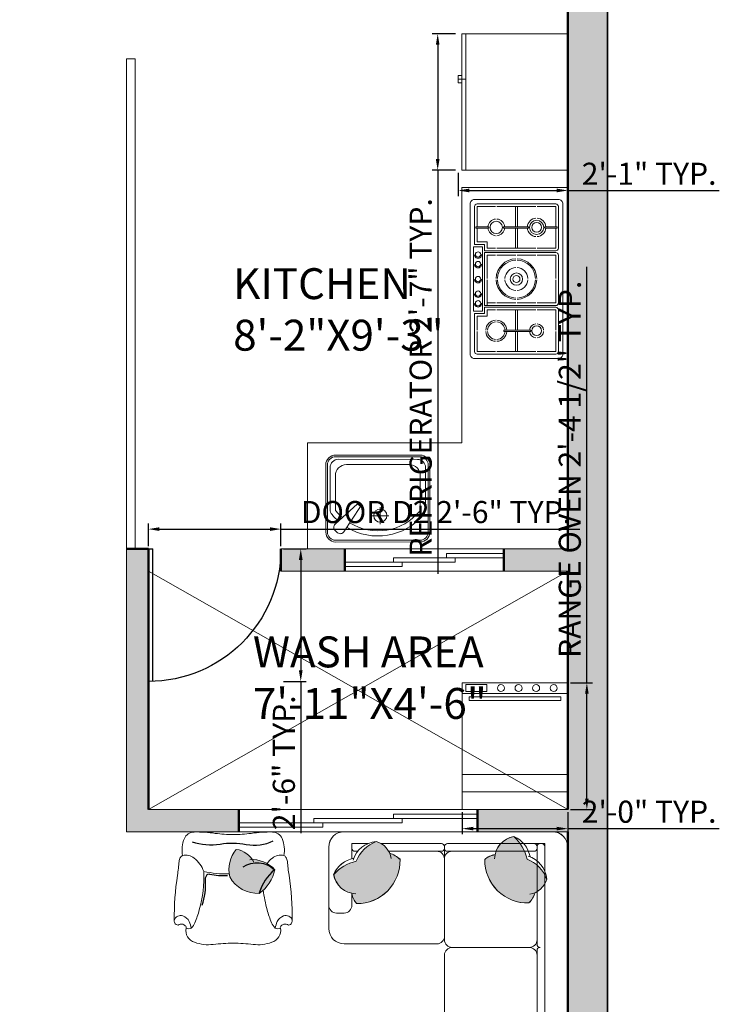
# Model space of a CAD drawing. Units: inches. Extents: x 1734 to 4011, y 1071 to 1891.
# Tile 4 of 27: x 1985 to 2144, y 1427 to 1650. Entities that reach past the tile are written whole.
import ezdxf

# ---------------------------------------------------------------- set-up
doc = ezdxf.new("R2010")
doc.units = ezdxf.units.IN
for name, color, linetype, lineweight in [('A-ANNO-DIMS', 2, 'Continuous', 18), ('A-AREA-IDEN', 3, 'Continuous', 18), ('A-DOOR', 3, 'Continuous', 25), ('A-EQPM', 8, 'Continuous', 18), ('A-FLOR-FIXT', 9, 'Continuous', 18), ('A-FURN', 8, 'Continuous', 18), ('A-FURN-PATT', 252, 'Continuous', 13), ('A-GLAZ', 4, 'Continuous', 18), ('A-WALL', 7, 'Continuous', 50), ('A-WALL-PATT', 8, 'Continuous', 13), ('C-PROP', 1, 'Continuous', 35)]:
    doc.layers.add(name, color=color, linetype=linetype, lineweight=lineweight)
doc.layers.add('IFF-FURN-DETAIL', color=250, linetype='Continuous')
doc.styles.get("Standard").update_dxf_attribs({"font": 'arial.ttf'})
doc.dimstyles.new('ISO-25', dxfattribs={"dimtxt": 5, "dimasz": 2.5, "dimexe": 1.25, "dimexo": 0.625, "dimtad": 1, "dimdec": 1, "dimlunit": 3, "dimtxsty": 'Standard', "dimcen": 2.5, "dimclrt": 1, "dimadec": 0, "dimazin": 0, "dimtfac": 1, "dimtdec": 1, "dimtmove": 0, "dimatfit": 3, "dimfxl": 1, "dimarcsym": 0})

# ---------------------------------------------------------------- blocks, each defined once
blk = doc.blocks.new('STOVE')
for p, q in [((11.85, 19.7), (11.55, 19.7)), ((11.55, 16.92), (11.55, 19.7)), ((11.85, 16.92), (11.85, 19.7)), ((11.85, 16.92), (11.55, 16.92)), ((-11.85, 13.73), (-11.85, 7.62)), ((-11.85, 13.73), (-11.55, 13.73)), ((-11.55, 13.73), (-11.55, 7.62)), ((11.85, 13.23), (11.55, 13.23)), ((11.55, 13.23), (11.55, 7.57)), ((11.85, 13.23), (11.85, 7.57)), ((-11.85, 10.75), (-16.4, 10.75)), ((-11.85, 10.25), (-16.4, 10.25)), ((-7, 10.75), (-11.55, 10.75)), ((-7, 10.25), (-11.55, 10.25)), ((7, 10.75), (11.55, 10.75)), ((7, 10.25), (11.55, 10.25)), ((11.85, 10.75), (16.4, 10.75)), ((11.85, 10.25), (16.4, 10.25)), ((-11.85, 7.62), (-11.55, 7.62)), ((11.85, 7.57), (11.55, 7.57)), ((-7, 3.9), (-8.4, 3.9)), ((-7.8, 3.3), (-7.8, 1)), ((-6.4, 3.3), (-7.8, 3.3)), ((7.3, 2.8), (-7.3, 2.8)), ((-7.3, 2.8), (-7.3, 0.8)), ((-5.4, 3.9), (-6, 3.9)), ((-5.4, 3.9), (-0.15, 3.9)), ((0.15, 3.9), (5.4, 3.9)), ((6.4, 3.3), (7.8, 3.3)), ((7, 3.9), (8.4, 3.9)), ((7.3, 2.8), (7.3, 0.8)), ((7.8, 3.3), (7.8, 1)), ((8.4, 3.9), (8.4, 1.6)), ((11.85, 4.28), (11.55, 4.28)), ((11.55, 4.28), (11.55, 1.3)), ((11.85, 4.28), (11.85, 1.3)), ((7.3, 0.8), (-7.3, 0.8)), ((11.85, 1.3), (11.55, 1.3))]:
    blk.add_line(p, q)
for points in [[(-17, 21), (17, 21, -0.414214), (18, 20), (18, 1, -0.414214), (17, 0), (-17, 0, -0.414214), (-18, 1), (-18, 20, -0.414214)], [(6, 3.3), (-6, 3.3), (-6, 19.4, -0.414214), (-5.4, 20), (5.4, 20, -0.414214), (6, 19.4)]]:
    blk.add_lwpolyline(points, format="xyb", close=True)
for points in [[(-7.8, 1), (-16.4, 1, -0.414214), (-17, 1.6), (-17, 19.4, -0.414214), (-16.4, 20), (-7, 20, -0.414214), (-6.4, 19.4), (-6.4, 3.3)], [(6.4, 19.4, -0.414214), (7, 20), (16.4, 20, -0.414214), (17, 19.4), (17, 1.6, -0.414214), (16.4, 1), (7.8, 1)]]:
    blk.add_lwpolyline(points, format="xyb")
for points in [[(-16.4, 15.22), (-16.4, 19.4), (-11.85, 19.4)], [(-11.55, 19.4), (-7, 19.4), (-7, 15.22)], [(-5.4, 15.22), (-5.4, 19.4), (-0.15, 19.4)], [(0.15, 19.4), (5.4, 19.4), (5.4, 15.22)], [(6.4, 3.3), (6.4, 19.4)], [(7, 15.22), (7, 19.4), (11.55, 19.4)], [(11.85, 19.4), (16.4, 19.4), (16.4, 15.22)], [(-16.4, 6.08), (-16.4, 14.92)], [(-7, 14.92), (-7, 6.08)], [(-5.4, 10.65), (-5.4, 14.92)], [(5.4, 14.92), (5.4, 10.65)], [(7, 6.08), (7, 14.92)], [(16.4, 14.92), (16.4, 6.08)], [(-5.4, 6.08), (-5.4, 10.35)], [(5.4, 10.35), (5.4, 6.08)], [(-11.85, 1.6), (-16.4, 1.6), (-16.4, 5.77)], [(-7, 5.77), (-7, 3.9)], [(-5.4, 3.9), (-5.4, 5.77)], [(5.4, 5.77), (5.4, 3.9)], [(7, 3.9), (7, 5.77)], [(16.4, 5.77), (16.4, 1.6), (11.85, 1.6)], [(-8.4, 3.9), (-8.4, 1.6), (-11.55, 1.6)], [(11.55, 1.6), (8.4, 1.6)]]:
    blk.add_lwpolyline(points)
for centre, radius in [((-11.7, 15.07), 1.1), ((11.7, 15.07), 1.6), ((11.7, 15.07), 1.1), ((0, 10.5), 1.4), ((0, 10.5), 0.8), ((11.7, 5.93), 1.4), ((-5.49, 1.8), 0.6), ((-3.3, 1.8), 0.6), ((0, 1.8), 0.6), ((3.39, 1.8), 0.6), ((5.57, 1.8), 0.6)]:
    blk.add_circle(centre, radius)
for centre, radius, start, end in [((-11.7, 15.07), 1.6, 95.3794, 174.6206), ((-11.7, 15.07), 1.6, 5.3794, 84.6206), ((11.7, 15.07), 2.1, 94.096, 175.904), ((11.7, 15.07), 2.1, 4.096, 85.904), ((-11.7, 15.07), 1.6, 185.3794, 264.6206), ((-11.7, 15.07), 1.6, 275.3794, 354.6206), ((0, 10.5), 4.6, 91.8687, 178.1313), ((0, 10.5), 4.3, 91.9991, 178.0009), ((0, 10.5), 4.6, 1.8687, 88.1313), ((0, 10.5), 4.3, 1.9991, 88.0009), ((11.7, 15.07), 2.1, 184.096, 265.904), ((11.7, 15.07), 2.1, 274.096, 355.904), ((0, 10.5), 2.6, 93.3074, 176.6926), ((0, 10.5), 2.6, 3.3074, 86.6926), ((0, 10.5), 4.6, 181.8687, 268.1313), ((0, 10.5), 4.3, 181.9991, 268.0009), ((0, 10.5), 2.6, 183.3074, 266.6926), ((0, 10.5), 4.6, 271.8687, 358.1313), ((0, 10.5), 4.3, 271.9991, 358.0009), ((0, 10.5), 2.6, 273.3074, 356.6926), ((-11.7, 5.93), 2.4, 93.5833, 176.4167), ((-11.7, 5.93), 2, 94.3012, 175.6988), ((-11.7, 5.93), 2.4, 3.5833, 86.4167), ((-11.7, 5.93), 2, 4.3012, 85.6988), ((11.7, 5.93), 1.9, 94.5281, 175.4719), ((11.7, 5.93), 1.9, 4.5281, 85.4719), ((-11.7, 5.93), 2.4, 183.5833, 266.4167), ((-11.7, 5.93), 2, 184.3012, 265.6988), ((-11.7, 5.93), 2.4, 273.5833, 356.4167), ((-11.7, 5.93), 2, 274.3012, 355.6988), ((11.7, 5.93), 1.9, 184.5281, 265.4719), ((11.7, 5.93), 1.9, 274.5281, 355.4719), ((-5.49, 1.8), 0.846, 89.9979, 270), ((-3.3, 1.8), 0.846, 89.9979, 270), ((0, 1.8), 0.846, 89.9979, 270), ((3.39, 1.8), 0.846, 89.9979, 270), ((5.57, 1.8), 0.846, 89.9979, 270)]:
    blk.add_arc(centre, radius, start, end)
blk = doc.blocks.new('Refrigerator-2 door - 36 in top')
for p, q in [((0, -26.999999), (36, -26.999999)), ((11, -27.999999), (11, -28.999999)), ((12, -26.999999), (12, -28.999999)), ((13, -28.999999), (13, -27.999999)), ((11, -28.999999), (13, -28.999999))]:
    blk.add_line(p, q)
blk.add_lwpolyline([(0, -27.999999), (0, 0), (36, 0), (36, -27.999999)], close=True)
blk = doc.blocks.new("D2 2'6")
for p, q in [((0, 30), (0, 0)), ((1, 30), (1, 0)), ((0, 0), (1, 0))]:
    blk.add_line(p, q)
blk.add_arc((0, 0), 30, 0, 90)
blk = doc.blocks.new('SOFA 1')
at = {"transparency": 33554687}
h = blk.add_hatch(color=256, dxfattribs=at)
h.dxf.hatch_style = 1
h.paths.add_polyline_path([(3723.52, 1308.63, 0.147724), (3717.76, 1305.24, 0.310469), (3722.42, 1300.4), (3722.42, 1300.25, 0.156703), (3723.62, 1297.8, 0.425821), (3734.69, 1309.08, 0.121928), (3732.05, 1310.63, 0.233216), (3728.6, 1313.59, 0.213835)])
h = blk.add_hatch(color=256, dxfattribs=at)
h.dxf.hatch_style = 1
h.paths.add_polyline_path([(3769.65, 1307.6, 0.084911), (3767.15, 1309.12, 0.046133), (3766.46, 1311.13), (3759.18, 1311.13, 0.039409), (3758.92, 1310.24, 0.165523), (3756.31, 1309.02, 0.42585), (3767.59, 1297.95, 0.121928), (3769.15, 1300.58, 0.027403), (3769.65, 1300.83)])
h.paths.add_polyline_path([(3765.34, 1313.08), (3760.4, 1313.08, 0.097704), (3759.18, 1311.13), (3766.46, 1311.13, 0.04873)])
h.paths.add_polyline_path([(3763.76, 1314.88, 0.16488), (3760.4, 1313.08), (3765.34, 1313.08, 0.051917)])
h.paths.add_polyline_path([(3771.6, 1305.17, 0.090388), (3769.65, 1307.6), (3769.65, 1300.83, 0.136035), (3771.6, 1302.77)])
h = blk.add_hatch(color=256, dxfattribs=at)
h.dxf.hatch_style = 1
h.paths.add_polyline_path([(3769.16, 1235.96, 0.122267), (3767.6, 1238.61, 0.425972), (3756.32, 1227.54, 0.165563), (3758.93, 1226.32, 0.309481), (3763.76, 1221.69, 0.002677), (3763.83, 1221.72, 0.146094), (3767.16, 1227.43, 0.212433), (3772.1, 1232.48, 0.235342)])
h = blk.add_hatch(color=256, dxfattribs=at)
h.dxf.hatch_style = 1
h.paths.add_polyline_path([(3769.16, 1225.36, 0.122267), (3767.6, 1228.01, 0.425972), (3756.32, 1216.94, 0.165563), (3758.93, 1215.72, 0.309481), (3763.76, 1211.09, 0.002677), (3763.83, 1211.12, 0.146094), (3767.16, 1216.83, 0.212433), (3772.1, 1221.88, 0.235342)])
for p, q in [((3720.45, 1316.13), (3773.58, 1316.13)), ((3777.51, 1312.19), (3777.51, 1213.72))]:
    blk.add_line(p, q, dxfattribs=at)
for points in [[(3717.76, 1305.24, -0.147724), (3723.52, 1308.63, -0.213355), (3728.59, 1313.59, 0.213355), (3723.52, 1308.63, 0.147724), (3717.76, 1305.24, -0.249545), (3722.86, 1309.34, 0.249545), (3717.75, 1305.25, 0.356779), (3723.4, 1300.28, -0.356779), (3717.76, 1305.24)], [(3728.58, 1313.6, -0.306333), (3732.42, 1309.31, 0.306333), (3728.58, 1313.6, 0.306674), (3722.72, 1308.89, -0.306674), (3728.58, 1313.6)], [(3763.76, 1314.88, -0.147724), (3767.15, 1309.12, -0.213355), (3772.1, 1304.05, 0.213355), (3767.15, 1309.12, 0.147724), (3763.76, 1314.88, -0.249545), (3767.86, 1309.77, 0.249545), (3763.77, 1314.89, 0.356779), (3758.8, 1309.23, -0.356779), (3763.76, 1314.88)], [(3734.69, 1309.08, -0.425972), (3723.62, 1297.8, -0.165552), (3722.4, 1300.4, 0.165552), (3723.62, 1297.79, 0.425972), (3734.69, 1309.07, 0.121514), (3732.07, 1310.63, -0.121514), (3734.69, 1309.08)], [(3767.6, 1297.95, -0.425972), (3756.31, 1309.01, -0.165552), (3758.92, 1310.24, 0.165552), (3756.31, 1309.02, 0.425972), (3767.59, 1297.95, 0.121514), (3769.14, 1300.57, -0.121514), (3767.6, 1297.95)], [(3772.11, 1304.06, -0.306333), (3767.83, 1300.22, 0.306333), (3772.11, 1304.06, 0.306674), (3767.4, 1309.91, -0.306674), (3772.11, 1304.06)], [(3770.44, 1286.63, -0.414214), (3769.66, 1287.4, 0.414214), (3770.44, 1286.63, 0.414214), (3769.66, 1285.83, -0.414214), (3770.44, 1286.63)], [(3748.01, 1262.99, -0.414214), (3746.05, 1264.95, 0.414214), (3748.01, 1262.97, 0.414213), (3746.05, 1261.01, -0.414213), (3748.01, 1262.99)], [(3770.44, 1262.99, -0.414214), (3769.66, 1263.77, 0.414214), (3770.44, 1262.99, 0.414214), (3769.66, 1262.19, -0.414214), (3770.44, 1262.99)], [(3770.83, 1262.97, -0.414214), (3771.61, 1262.19, 0.414214), (3770.83, 1262.99, 0.414214), (3771.61, 1263.77, -0.414214), (3770.83, 1262.97)], [(3748.01, 1239.35, -0.414214), (3746.05, 1241.31, 0.414214), (3748.01, 1239.33, 0.414213), (3746.05, 1237.37, -0.414213), (3748.01, 1239.35)], [(3767.7, 1239.33, -0.414214), (3769.66, 1237.37, 0.414214), (3767.7, 1239.35, 0.414214), (3769.66, 1241.31, -0.414214), (3767.7, 1239.33)], [(3756.32, 1227.54, -0.425972), (3767.6, 1238.61, -0.121514), (3769.16, 1235.98, 0.121514), (3767.6, 1238.61, 0.425972), (3756.32, 1227.54, 0.165552), (3758.93, 1226.32, -0.165552), (3756.32, 1227.54)], [(3770.44, 1239.35, -0.414214), (3769.66, 1240.13, 0.414214), (3770.44, 1239.33, 0.414214), (3769.66, 1238.55, -0.414214), (3770.44, 1239.35)], [(3770.83, 1239.33, -0.414214), (3771.61, 1238.55, 0.414214), (3770.83, 1239.35, 0.414214), (3771.61, 1240.13, -0.414214), (3770.83, 1239.33)], [(3772.1, 1232.5, -0.306674), (3767.41, 1226.64, 0.306674), (3772.1, 1232.5, 0.306333), (3767.84, 1236.34, -0.306333), (3772.1, 1232.5)], [(3763.78, 1221.67, 0.249545), (3767.87, 1226.78, -0.249545), (3763.76, 1221.69, -0.356779), (3758.81, 1227.32, 0.356779), (3763.77, 1221.68, 0.147724), (3767.16, 1227.43, 0.213355), (3772.11, 1232.51, -0.213355), (3767.16, 1227.43, -0.147724), (3763.78, 1221.67)], [(3756.32, 1216.94, -0.200233), (3759.49, 1224.76, 0.200233), (3756.32, 1216.94, 0.165552), (3758.93, 1215.72, -0.165552), (3756.32, 1216.94)], [(3772.1, 1221.9, -0.306674), (3767.41, 1216.04, 0.306674), (3772.1, 1221.9, -0.213355), (3767.16, 1216.83, -0.147724), (3763.77, 1211.08, 0.147724), (3767.15, 1216.83, 0.213355), (3772.1, 1221.9)], [(3763.76, 1211.09, -0.356779), (3758.81, 1216.72, 0.356779), (3763.76, 1211.09, 0.249545), (3767.87, 1216.18, -0.249545), (3763.76, 1211.09)]]:
    blk.add_lwpolyline(points, format="xyb", dxfattribs=at)
for points in [[(3716.51, 1312.2), (3716.51, 1291.44)], [(3722.42, 1313.08), (3722.42, 1309.23), (3722.42, 1313.08), (3726.57, 1313.08)], [(3723.21, 1311.13), (3723.93, 1311.13)], [(3729.85, 1313.08), (3745.25, 1313.08)], [(3731.82, 1311.13), (3745.25, 1311.13)], [(3746.01, 1312.3), (3746.01, 1288.55)], [(3746.01, 1310.97), (3746.01, 1311.36)], [(3768.11, 1313.08), (3746.78, 1313.08)], [(3768.87, 1311.13), (3746.78, 1311.13)], [(3771.6, 1313.08), (3767.75, 1313.08), (3771.6, 1313.08), (3771.6, 1308.93)], [(3769.66, 1287.39), (3769.65, 1312.3)], [(3771.6, 1313.08), (3771.61, 1233.74)], [(3769.65, 1309.43), (3769.65, 1308.71)], [(3746.01, 1288.54), (3746.01, 1308.23)], [(3722.42, 1300.39), (3722.42, 1297.33)], [(3720.45, 1295.38), (3718.48, 1295.38)], [(3720.45, 1287.5), (3744.09, 1287.5)], [(3747.99, 1286.6), (3767.69, 1286.6)], [(3769.66, 1263.75), (3769.66, 1285.81)], [(3746.02, 1284.63), (3746.02, 1264.94)], [(3769.66, 1277.18), (3769.66, 1263.75)], [(3746.02, 1260.99), (3746.02, 1241.3)], [(3747.99, 1262.97), (3767.69, 1262.97)], [(3769.66, 1240.12), (3769.66, 1262.18)], [(3770.43, 1262.97), (3770.82, 1262.97)], [(3747.99, 1239.33), (3767.69, 1239.33)], [(3769.66, 1235.71), (3769.66, 1238.54)], [(3770.43, 1239.33), (3770.82, 1239.33)], [(3746.02, 1237.36), (3746.02, 1213.74)], [(3771.61, 1223.14), (3771.61, 1230.47)], [(3769.66, 1225.11), (3769.66, 1227.82)], [(3767.76, 1215.72), (3771.61, 1215.72), (3771.61, 1219.84), (3771.61, 1215.72)], [(3755.86, 1215.72), (3758.92, 1215.72)], [(3769.66, 1216.5), (3769.66, 1217.22)], [(3753.91, 1211.77), (3753.91, 1213.74)], [(3749.97, 1209.8), (3773.58, 1209.8)]]:
    blk.add_lwpolyline(points, close=True, dxfattribs=at)
for points in [[(3722.42, 1311.91, 0.414214), (3723.2, 1311.13, -0.414214)], [(3770.43, 1313.08, 0.414214), (3769.65, 1312.3, -0.414214)], [(3771.6, 1312.3, 0.414214), (3770.82, 1313.08, -0.414214)], [(3716.51, 1297.34, 0.414214), (3718.47, 1295.38, -0.414214)], [(3720.44, 1295.38, 0.414214), (3722.4, 1297.34, -0.414214)], [(3716.51, 1291.45, 0.414212), (3720.44, 1287.52, -0.414212)], [(3746.03, 1288.56, 0.414214), (3747.99, 1286.6, 0.414213), (3746.03, 1284.64, -0.414213), (3747.99, 1286.6, -0.414214)], [(3769.66, 1284.64, 0.414214), (3767.7, 1286.6, 0.414214), (3769.66, 1288.56, -0.414214), (3767.7, 1286.6, -0.414214)], [(3769.66, 1261.01, 0.414214), (3767.7, 1262.97, 0.414214), (3769.66, 1264.93, -0.414214), (3767.7, 1262.97, -0.414214)], [(3772.13, 1221.9, 0.306333), (3767.84, 1225.74, -0.306333)], [(3769.16, 1225.36, 0.071861), (3768.39, 1227.01, -0.071861)], [(3755.87, 1215.72, 0.414214), (3753.91, 1213.76, -0.414214)], [(3769.66, 1216.52, 0.414214), (3770.44, 1215.74, -0.414214)], [(3770.83, 1215.74, 0.414214), (3771.61, 1216.52, -0.414214)], [(3746.05, 1213.76, 0.414212), (3749.98, 1209.82, -0.414212)], [(3755.87, 1209.8, -0.414214), (3753.91, 1211.76, 0.414214)]]:
    blk.add_lwpolyline(points, format="xyb", close=True, dxfattribs=at)
for centre, radius, start, end in [((3720.44, 1312.2), 3.93, 90.0002, 179.9998), ((3720.44, 1312.19), 3.94, 89.9158, 179.9154), ((3773.58, 1312.2), 3.93, 0.0002, 89.9998), ((3773.57, 1312.19), 3.94, 359.9158, 89.9154), ((3744.09, 1309.21), 1.92, 358.766, 90.5111), ((3745.22, 1312.29), 0.789, 0.8425, 90.8425), ((3745.24, 1311.91), 0.777, 270, 0), ((3745.24, 1311.91), 0.777, 270, 0), ((3746.8, 1312.29), 0.789, 89.1575, 179.1575), ((3746.79, 1311.91), 0.777, 180, 270), ((3746.79, 1311.91), 0.777, 180, 270), ((3747.93, 1309.21), 1.92, 89.4889, 181.234), ((3768.87, 1312.3), 0.777, 360, 90), ((3768.87, 1311.91), 0.777, 270, 0), ((3744.08, 1289.48), 1.96, 270, 360), ((3744.08, 1289.48), 1.96, 270, 360), ((3773.58, 1213.73), 3.93, 270.0002, 359.9998), ((3773.59, 1213.73), 3.93, 269.9156, 359.9152)]:
    blk.add_arc(centre, radius, start, end, dxfattribs=at)
blk = doc.blocks.new('PILLOW-1')
at = {"color": 0}
blk.add_lwpolyline([(198, -165.3, -0.232884), (126.3, -346, -0.184752), (-44.3, -233.7, -0.286563), (74.8, -22, -0.237978), (272.6, -68.2, -0.243587), (179.4, -195.4, 4.263709)], format="xyb", dxfattribs=at)
at = {"layer": 'IFF-FURN-DETAIL'}
blk.add_lwpolyline([(147.6, -117.6, -0.343333), (126.5, -342.2, 0.126408), (-39.5, -232.6, -5.969376)], format="xyb", dxfattribs=at)
blk = doc.blocks.new('CLNG90')
for points in [[(689.4, 369.7, 0.157831), (676.6, 385.2, 0.121013), (646.4, 395.4, -0.017334), (546.8, 407.4, 0.041496), (215.3, 431.2, 0.153531), (191.4, 423.4, 0.382906), (185.1, 395.3, -0.284047), (183.7, 360.8, 0.011997), (177.2, 350.7, -0.370479), (159.9, 345, 0.380647), (56.2, 282, 0.117468), (40.6, 145.8, -0.027775), (50, 0, -8.773898)], [(159.9, 345, 0.22481), (159.8, 306.3, 0.055398), (209.2, 321.6, 0.180116), (248.9, 368.2, 0.194833), (247.6, 405.4, 0.242377), (215.3, 431.2, 1.52074)], [(159.9, 345, 0.22481), (159.8, 306.3, 0.055398), (209.2, 321.6, 0.180116), (248.9, 368.2, 0.194833), (247.6, 405.4, 0.242377), (215.3, 431.2, 1.52074)], [(689.4, 369.7, -0.235486), (671.3, 286, -0.134038), (573.9, 215.1, -0.079303), (292.9, 247.8, -0.027048), (199.2, 279.7, -0.106276), (159.8, 306.3, -1.699)], [(689.4, 369.7, -0.235486), (671.3, 286, -0.134038), (573.9, 215.1, -0.079303), (292.9, 247.8, -0.027048), (199.2, 279.7, -0.106276), (159.8, 306.3, -1.699)], [(689.4, 369.7, -0.146607), (813.9, 357.3, -0.305296), (861.7, 285.6, -0.042137), (851.9, 131.4, 0.040285), (843.1, 0, 3.952121)], [(573.9, 215.1, 0.061244), (555.6, 29, 3.376255)], [(573.9, 215.1, 0.061244), (555.6, 29, 3.376255)], [(689.4, -369.7, -0.157831), (676.6, -385.2, -0.121013), (646.4, -395.4, 0.017334), (546.8, -407.4, -0.041496), (215.3, -431.2, -0.153531), (191.4, -423.4, -0.382906), (185.1, -395.3, 0.284047), (183.7, -360.8, -0.011997), (177.2, -350.7, 0.370479), (159.9, -345, -0.380647), (56.2, -282, -0.117468), (40.6, -145.8, 0.027775), (50, 0, 8.773898)], [(689.4, -369.7, 0.146607), (813.9, -357.3, 0.305296), (861.7, -285.6, 0.042137), (851.9, -131.4, -0.040285), (843.1, 0, -3.952121)], [(437.4, -219.7, 0.041086), (292.9, -247.8, 0.027048), (199.2, -279.7, 0.106276), (159.8, -306.3, 1.699)], [(437.4, -219.7, 0.041086), (292.9, -247.8, 0.027048), (199.2, -279.7, 0.106276), (159.8, -306.3, 1.699)], [(689.4, -369.7, 0.235486), (671.3, -286, 0.060693), (631.8, -247.3, 0.001296)], [(689.4, -369.7, 0.235486), (671.3, -286, 0.060693), (631.8, -247.3, 0.001296)], [(159.9, -345, -0.22481), (159.8, -306.3, -0.055398), (209.2, -321.6, -0.180116), (248.9, -368.2, -0.194833), (247.6, -405.4, -0.242377), (215.3, -431.2, -1.52074)], [(159.9, -345, -0.22481), (159.8, -306.3, -0.055398), (209.2, -321.6, -0.180116), (248.9, -368.2, -0.194833), (247.6, -405.4, -0.242377), (215.3, -431.2, -1.52074)]]:
    blk.add_lwpolyline(points, format="xyb")
at = {"layer": 'IFF-FURN-DETAIL'}
for points in [[(790.6, 301.1, 0.124986), (773.9, 95.7, -0.091334), (771.1, -94.9, 0.164688), (796.9, -292.4, 1.068868)], [(790.6, 301.1, 0.124986), (773.9, 95.7, -0.091334), (771.1, -94.9, 0.164688), (796.9, -292.4, 1.068868)], [(328.2, 228.3, 0.109125), (508.5, 203.4, -0.16587), (546, 193.9, -0.314359), (554.8, 172.3, 0.072017), (544.2, 42.1, 4.351186)], [(328.2, 228.3, 0.109125), (508.5, 203.4, -0.16587), (546, 193.9, -0.314359), (554.8, 172.3, 0.072017), (544.2, 42.1, 4.351186)]]:
    blk.add_lwpolyline(points, format="xyb", dxfattribs=at)
at = {"xscale": 1.016, "yscale": 1.016, "zscale": 1.016}
blk.add_blockref('PILLOW-1', (458.1, 47.3), dxfattribs=at)
blk.add_blockref('PILLOW-1', (458.1, 47.3), dxfattribs=at)
blk = doc.blocks.new('Range-Oven - 30 in front')
for p, q in [((0, 33.00005), (30, 33.00005)), ((30, 10), (0, 10)), ((0, 5), (30, 5))]:
    blk.add_line(p, q)
for points in [[(0, 0), (0, 36.00005), (30, 36.00005), (30, 0)], [(1, 33.50005), (1, 35.50005), (7, 35.50005), (7, 33.50005)], [(2, 31.00005), (2, 32.00005), (28, 32.00005), (28, 31.00005)]]:
    blk.add_lwpolyline(points, close=True)
for centre in [(11, 34.50005), (16, 34.50005), (21, 34.50005), (26, 34.50005)]:
    blk.add_circle(centre, 1)
blk = doc.blocks.new('*D71')
at = {"layer": 'A-ANNO-DIMS', "color": 0, "lineweight": -2, "transparency": 16777216}
for p, q in [((2014.65, 1530.69), (2014.65, 1535.81)), ((2017.15, 1534.56), (2042.15, 1534.56)), ((2044.65, 1530.69), (2044.65, 1535.81)), ((2044.65, 1534.56), (2112.39, 1534.56))]:
    blk.add_line(p, q, dxfattribs=at)
at = {"layer": 'A-ANNO-DIMS', "color": 0, "transparency": 16777216}
for points in [[(2017.15, 1534.98), (2017.15, 1534.14), (2014.65, 1534.56)], [(2042.15, 1534.98), (2042.15, 1534.14), (2044.65, 1534.56)]]:
    blk.add_solid(points, dxfattribs=at)
at = {"layer": 'Defpoints', "color": 0, "transparency": 16777216}
for p in [(2044.65, 1534.56), (2014.65, 1530.06), (2044.65, 1530.06)]:
    blk.add_point(p, dxfattribs=at)
at = {"layer": 'A-ANNO-DIMS', "color": 1, "transparency": 16777216, "insert": (2079.77, 1537.77), "char_height": 5, "attachment_point": 5}
blk.add_mtext('DOOR D2 2\'-6" TYP.', dxfattribs=at)
blk = doc.blocks.new('*D72')
at = {"layer": 'A-ANNO-DIMS', "color": 0, "lineweight": -2, "transparency": 16777216}
for p, q in [((2045.27, 1530.06), (2050.4, 1530.06)), ((2049.15, 1527.56), (2049.15, 1502.56)), ((2045.27, 1500.06), (2050.4, 1500.06)), ((2049.15, 1500.06), (2049.15, 1465.75))]:
    blk.add_line(p, q, dxfattribs=at)
at = {"layer": 'A-ANNO-DIMS', "color": 0, "transparency": 16777216}
for points in [[(2048.73, 1527.56), (2049.57, 1527.56), (2049.15, 1530.06)], [(2048.73, 1502.56), (2049.57, 1502.56), (2049.15, 1500.06)]]:
    blk.add_solid(points, dxfattribs=at)
at = {"layer": 'Defpoints', "color": 0, "transparency": 16777216}
for p in [(2044.65, 1530.06), (2044.65, 1500.06), (2049.15, 1500.06)]:
    blk.add_point(p, dxfattribs=at)
at = {"layer": 'A-ANNO-DIMS', "color": 1, "transparency": 16777216, "insert": (2045.97, 1481.65), "char_height": 5, "attachment_point": 5, "rotation": 90}
blk.add_mtext('2\'-6" TYP.', dxfattribs=at)
blk = doc.blocks.new('*D97')
at = {"layer": 'A-ANNO-DIMS', "color": 0, "lineweight": -2, "transparency": 16777216}
for p, q in [((2084.17, 1646.7), (2078.92, 1646.7)), ((2080.17, 1644.2), (2080.17, 1618.35)), ((2084.17, 1615.85), (2078.92, 1615.85)), ((2080.17, 1615.85), (2080.17, 1524.45))]:
    blk.add_line(p, q, dxfattribs=at)
at = {"layer": 'A-ANNO-DIMS', "color": 0, "transparency": 16777216}
for points in [[(2079.75, 1644.2), (2080.59, 1644.2), (2080.17, 1646.7)], [(2079.75, 1618.35), (2080.59, 1618.35), (2080.17, 1615.85)]]:
    blk.add_solid(points, dxfattribs=at)
at = {"layer": 'Defpoints', "color": 0, "transparency": 16777216}
for p in [(2084.8, 1646.7), (2080.17, 1615.85), (2084.8, 1615.85)]:
    blk.add_point(p, dxfattribs=at)
at = {"layer": 'A-ANNO-DIMS', "color": 1, "transparency": 16777216, "insert": (2076.96, 1568.9), "char_height": 5, "attachment_point": 5, "rotation": 90}
blk.add_mtext('REFRIGERATOR 2\'-7" TYP.', dxfattribs=at)
blk = doc.blocks.new('*D98')
at = {"layer": 'A-ANNO-DIMS', "color": 0, "lineweight": -2, "transparency": 16777216}
for p, q in [((2084.8, 1615.23), (2084.8, 1609.97)), ((2109.65, 1615.23), (2109.65, 1609.97)), ((2087.3, 1611.22), (2107.15, 1611.22)), ((2109.65, 1611.22), (2143.96, 1611.22))]:
    blk.add_line(p, q, dxfattribs=at)
at = {"layer": 'A-ANNO-DIMS', "color": 0, "transparency": 16777216}
for points in [[(2087.3, 1611.64), (2087.3, 1610.81), (2084.8, 1611.22)], [(2107.15, 1611.64), (2107.15, 1610.81), (2109.65, 1611.22)]]:
    blk.add_solid(points, dxfattribs=at)
at = {"layer": 'Defpoints', "color": 0, "transparency": 16777216}
for p in [(2084.8, 1615.85), (2109.65, 1615.85), (2109.65, 1611.22)]:
    blk.add_point(p, dxfattribs=at)
at = {"layer": 'A-ANNO-DIMS', "color": 1, "transparency": 16777216, "insert": (2128.06, 1614.36), "char_height": 5, "attachment_point": 5}
blk.add_mtext('2\'-1" TYP.', dxfattribs=at)
blk = doc.blocks.new('*D101')
at = {"layer": 'A-ANNO-DIMS', "color": 0, "lineweight": -2, "transparency": 16777216}
for p, q in [((2113.96, 1499.77), (2113.96, 1593.91)), ((2110.27, 1499.77), (2115.21, 1499.77)), ((2113.96, 1473.56), (2113.96, 1497.27)), ((2110.27, 1471.06), (2115.21, 1471.06))]:
    blk.add_line(p, q, dxfattribs=at)
at = {"layer": 'A-ANNO-DIMS', "color": 0, "transparency": 16777216}
for points in [[(2113.54, 1497.27), (2114.37, 1497.27), (2113.96, 1499.77)], [(2113.54, 1473.56), (2114.37, 1473.56), (2113.96, 1471.06)]]:
    blk.add_solid(points, dxfattribs=at)
at = {"layer": 'Defpoints', "color": 0, "transparency": 16777216}
for p in [(2109.65, 1499.77), (2113.96, 1499.77), (2109.65, 1471.06)]:
    blk.add_point(p, dxfattribs=at)
at = {"layer": 'A-ANNO-DIMS', "color": 1, "transparency": 16777216, "insert": (2110.74, 1548.09), "char_height": 5, "attachment_point": 5, "rotation": 90}
blk.add_mtext('RANGE OVEN 2\'-4 1/2" TYP.', dxfattribs=at)
blk = doc.blocks.new('*D102')
at = {"layer": 'A-ANNO-DIMS', "color": 0, "lineweight": -2, "transparency": 16777216}
for p, q in [((2085.72, 1470.44), (2085.72, 1465.5)), ((2109.65, 1470.44), (2109.65, 1465.5)), ((2088.22, 1466.75), (2107.15, 1466.75)), ((2109.65, 1466.75), (2143.96, 1466.75))]:
    blk.add_line(p, q, dxfattribs=at)
at = {"layer": 'A-ANNO-DIMS', "color": 0, "transparency": 16777216}
for points in [[(2088.22, 1467.17), (2088.22, 1466.34), (2085.72, 1466.75)], [(2107.15, 1467.17), (2107.15, 1466.34), (2109.65, 1466.75)]]:
    blk.add_solid(points, dxfattribs=at)
at = {"layer": 'Defpoints', "color": 0, "transparency": 16777216}
for p in [(2085.72, 1471.06), (2109.65, 1471.06), (2109.65, 1466.75)]:
    blk.add_point(p, dxfattribs=at)
at = {"layer": 'A-ANNO-DIMS', "color": 1, "transparency": 16777216, "insert": (2128.06, 1469.93), "char_height": 5, "attachment_point": 5}
blk.add_mtext('2\'-0" TYP.', dxfattribs=at)

msp = doc.modelspace()

# ---------------------------------------------------------------- hatches: boundary and pattern name
at = {"layer": 'A-FURN-PATT'}
h = msp.add_hatch(color=256, dxfattribs=at)
h.dxf.hatch_style = 1
h.paths.add_polyline_path([(2039.75, 1452.08, 0.184752), (2043.29, 1457.45, 0.210353), (2038.19, 1459.73, 0.209279), (2034.54, 1462.06, 0.237978), (2033.08, 1455.83, 0.286563)])
at = {"layer": 'A-WALL-PATT'}
h = msp.add_hatch(color=256, dxfattribs=at)
h.dxf.hatch_style = 1
h.paths.add_polyline_path([(1857.65, 1835.06), (1857.65, 1793.06), (1862.65, 1793.06), (1862.65, 1835.06), (1951.65, 1835.06), (1951.65, 1763.06), (1897.65, 1763.06), (1897.65, 1758.06), (1951.65, 1758.06), (1951.65, 1617.06), (1956.65, 1617.06), (1956.65, 1758.06), (2009.65, 1758.06), (2009.65, 1763.06), (1956.65, 1763.06), (1956.65, 1835.06), (2044.65, 1835.06), (2044.65, 1763.06), (2039.65, 1763.06), (2039.65, 1758.06), (2054.65, 1758.06), (2054.65, 1763.06), (2049.65, 1763.06), (2049.65, 1835.06), (2109.65, 1835.06), (2109.65, 1763.06), (2084.65, 1763.06), (2084.65, 1758.06), (2109.65, 1758.06), (2109.65, 1530.06), (2095.15, 1530.06), (2095.15, 1525.06), (2109.65, 1525.06), (2109.65, 1471.06), (2089.15, 1471.06), (2089.15, 1466.06), (2109.65, 1466.06), (2109.65, 1250.06), (2015.65, 1250.06), (2015.65, 1241.06), (2109.65, 1241.06), (2109.65, 1133.06), (1952.65, 1133.06), (1952.65, 1197.06), (1953.65, 1197.06), (1953.65, 1202.06), (1946.65, 1202.06), (1946.65, 1133.06), (1934.65, 1133.06), (1934.65, 1124.06), (2118.65, 1124.06), (2118.65, 1844.06), (1758.65, 1844.06), (1758.65, 1758.06), (1773.65, 1758.06), (1773.65, 1763.06), (1767.65, 1763.06), (1767.65, 1835.06)])
h.paths.add_polyline_path([(1803.65, 1649.06), (1812.65, 1649.06), (1812.65, 1758.06), (1867.65, 1758.06), (1867.65, 1763.06), (1797.65, 1763.06), (1797.65, 1758.06), (1803.65, 1758.06)], flags=17)
h.paths.add_polyline_path([(1803.65, 1572.06), (1956.65, 1572.06), (1956.65, 1581.06), (1951.65, 1581.06), (1951.65, 1577.06), (1812.65, 1577.06), (1812.65, 1601.06), (1803.65, 1601.06)], flags=17)
h.paths.add_polyline_path([(2044.65, 1530.06), (2044.65, 1525.06), (2059.15, 1525.06), (2059.15, 1530.06)], flags=17)
h.paths.add_polyline_path([(2009.65, 1466.06), (2035.15, 1466.06), (2035.15, 1471.06), (2014.65, 1471.06), (2014.65, 1530.06), (2009.65, 1530.06)], flags=17)
h.paths.add_polyline_path([(1896.65, 1537.06), (1896.65, 1533.06), (1901.65, 1533.06), (1901.65, 1542.06), (1803.65, 1542.06), (1803.65, 1507.06), (1812.65, 1507.06), (1812.65, 1537.06)], flags=17)
h.paths.add_polyline_path([(1906.65, 1466.06), (1906.65, 1471.06), (1901.65, 1471.06), (1901.65, 1503.06), (1896.65, 1503.06), (1896.65, 1471.06), (1812.65, 1471.06), (1812.65, 1483.06), (1803.65, 1483.06), (1803.65, 1400.06), (1812.65, 1400.06), (1812.65, 1466.06)], flags=17)
h.paths.add_polyline_path([(1951.65, 1334.06), (1909.15, 1334.06), (1909.15, 1325.06), (1956.65, 1325.06), (1956.65, 1466.06), (1961.65, 1466.06), (1961.65, 1471.06), (1942.65, 1471.06), (1942.65, 1466.06), (1951.65, 1466.06)], flags=17)
h.paths.add_polyline_path([(1812.65, 1334.06), (1812.65, 1352.06), (1803.65, 1352.06), (1803.65, 1325.06), (1855.15, 1325.06), (1855.15, 1334.06)], flags=17)
h.paths.add_polyline_path([(1956.65, 1298.06), (1956.65, 1301.06), (1947.65, 1301.06), (1947.65, 1298.06)], flags=17)
h.paths.add_polyline_path([(1967.65, 1241.06), (1967.65, 1250.06), (1947.65, 1250.06), (1947.65, 1241.06)], flags=17)

# ---------------------------------------------------------------- linework, layer by layer
at = {"layer": 'A-FLOR-FIXT'}
msp.add_circle((2067.17, 1537.61), 1.5, dxfattribs=at)
at = {"layer": 'A-FURN'}
for p, q in [((2009.65, 1641.06), (2009.65, 1466.06)), ((2009.65, 1641.06), (2011.65, 1641.06)), ((2011.65, 1641.06), (2011.65, 1530.06)), ((2085.65, 1611.93), (2109.65, 1611.93)), ((2085.65, 1611.93), (2085.65, 1554.06)), ((2050.65, 1554.06), (2085.65, 1554.06)), ((2050.65, 1554.06), (2050.65, 1530.06)), ((2044.65, 1530.06), (2109.65, 1530.06)), ((2109.65, 1525.06), (2014.65, 1471.06)), ((2014.65, 1525.06), (2109.65, 1471.06)), ((2044.65, 1525.06), (2109.65, 1525.06)), ((2014.65, 1471.06), (2109.65, 1471.06)), ((2009.65, 1466.06), (2109.65, 1466.06))]:
    msp.add_line(p, q, dxfattribs=at)
for points in [[(2057.05, 1551.33, 0.414214), (2054.82, 1549.11), (2054.84, 1533.88, 0.414214), (2057.04, 1531.64), (2076.19, 1531.66, 0.414214), (2078.41, 1533.87), (2078.41, 1549.11, 0.414214), (2076.18, 1551.33), (2057.05, 1551.33)], [(2057.05, 1550.96, 0.414214), (2055.21, 1549.11), (2055.21, 1533.88, 0.414214), (2057.04, 1532.03), (2076.19, 1532.03, 0.414214), (2078.01, 1533.87), (2078.01, 1549.11, 0.414214), (2076.18, 1550.94), (2057.05, 1550.96)], [(2059.57, 1534.99, 0.371519), (2077, 1537.84, 0.175764), (2077.41, 1539.02), (2077.43, 1548.51, 0.414214), (2075.58, 1550.33), (2057.66, 1550.36, 0.414214), (2055.81, 1548.5), (2055.81, 1539.02, 0.175764), (2056.24, 1537.84, 0.038632), (2057.7, 1536.36)], [(2060.23, 1535.97, 0.370401), (2076.09, 1538.6, 0.175764), (2076.23, 1539.02), (2076.23, 1546.66, 0.414214), (2073.72, 1549.15), (2059.51, 1549.15, 0.414214), (2057, 1546.65), (2057, 1539.02, 0.175764), (2057.15, 1538.6, 0.038512), (2058.59, 1537.16)]]:
    msp.add_lwpolyline(points, format="xyb", dxfattribs=at)
msp.add_lwpolyline([(2056.93, 1534.24), (2057.51, 1533.75, 0.463205), (2058.9, 1533.96), (2062.72, 1539.69), (2062.03, 1540.29), (2056.95, 1535.65, 0.4637)], format="xyb", close=True, dxfattribs=at)
for points in [[(2067.16, 1535.65), (2067.16, 1539.55)], [(2069.1, 1537.6), (2065.21, 1537.6)]]:
    msp.add_lwpolyline(points, dxfattribs=at)
at = {"layer": 'A-GLAZ'}
for p, q in [((2059.15, 1527.06), (2084.15, 1527.06)), ((2070.15, 1528.06), (2095.15, 1528.06)), ((2070.15, 1527.06), (2070.15, 1528.06)), ((2072.15, 1526.06), (2072.15, 1527.06)), ((2082.15, 1529.06), (2095.15, 1529.06)), ((2082.15, 1528.06), (2082.15, 1529.06)), ((2084.15, 1527.06), (2084.15, 1528.06)), ((2059.15, 1526.06), (2072.15, 1526.06)), ((2052.15, 1469.06), (2052.15, 1468.06)), ((2052.15, 1469.06), (2089.15, 1469.06)), ((2070.15, 1470.06), (2070.15, 1469.06)), ((2070.15, 1470.06), (2089.15, 1470.06)), ((2072.15, 1469.06), (2072.15, 1468.06)), ((2035.15, 1468.06), (2072.15, 1468.06)), ((2035.15, 1467.06), (2054.15, 1467.06)), ((2054.15, 1468.06), (2054.15, 1467.06))]:
    msp.add_line(p, q, dxfattribs=at)
at = {"layer": 'A-WALL'}
for p, q in [((2109.65, 1758.06), (2109.65, 1530.06)), ((2009.65, 1530.06), (2014.65, 1530.06)), ((2014.65, 1530.06), (2014.65, 1471.06)), ((2044.65, 1530.06), (2044.65, 1525.06)), ((2059.15, 1525.06), (2059.15, 1530.06)), ((2095.15, 1525.06), (2095.15, 1530.06)), ((2109.65, 1525.06), (2109.65, 1471.06)), ((2035.15, 1471.06), (2035.15, 1466.06)), ((2089.15, 1471.06), (2089.15, 1466.06)), ((2109.65, 1466.06), (2109.65, 1250.06))]:
    msp.add_line(p, q, dxfattribs=at)
at = {"layer": 'C-PROP'}
msp.add_lwpolyline([(1814.65, 1124.06), (1758.65, 1124.06), (1758.65, 1844.06), (2118.65, 1844.06), (2118.65, 1124.06), (1934.65, 1124.06)], dxfattribs=at)

# ---------------------------------------------------------------- block references
at = {"layer": 'A-DOOR', "xscale": -1, "rotation": 180}
msp.add_blockref("D2 2'6", (2014.65, 1530.06), dxfattribs=at)
at = {"layer": 'A-EQPM', "xscale": 0.8569942030484906, "yscale": 0.8569942030484906, "zscale": 0.8569942030484906, "rotation": 270}
msp.add_blockref('Refrigerator-2 door - 36 in top', (2109.65, 1646.7), dxfattribs=at)
at = {"layer": 'A-EQPM', "xscale": -1, "rotation": 270}
msp.add_blockref('STOVE', (2087.51, 1591.17), dxfattribs=at)
at = {"layer": 'A-EQPM', "xscale": 0.7975329364922055, "yscale": 0.7975329364922055, "zscale": 0.7975329364922055}
msp.add_blockref('Range-Oven - 30 in front', (2085.72, 1471.06), dxfattribs=at)
at = {"layer": 'A-FURN', "xscale": 0.031001591544, "yscale": 0.031001591544, "zscale": 0.031001591544, "rotation": 90}
msp.add_blockref('CLNG90', (2033.86, 1439.27), dxfattribs=at)
at = {"layer": 'A-FURN', "xscale": 0.887653230693335, "yscale": 0.887653230693335, "zscale": 0.887653230693335}
msp.add_blockref('SOFA 1', (-1243.47, 297.79), dxfattribs=at)

# ---------------------------------------------------------------- texts
at = {"layer": 'A-AREA-IDEN', "char_height": 7, "attachment_point": 1}
for s, insert in [('KITCHEN\\P8\'-2"X9\'-3"', (2033.85, 1593.63)), ('WASH AREA\\P7\'-11"X4\'-6"', (2038.32, 1510.26))]:
    msp.add_mtext_dynamic_manual_height_columns(s, width=86.9528, gutter_width=12.5, heights=[0], dxfattribs=dict(at, insert=insert))

# ---------------------------------------------------------------- dimensions: what is measured, and where the dimension line sits
at = {"layer": 'A-ANNO-DIMS'}
for base, p1, p2, angle, text, picture, middle in [((2080.1689, 1615.8503), (2084.7967, 1646.7021), (2084.7967, 1615.8503), 270, 'REFRIGERATOR <> TYP.', '*D97', (2076.9569, 1568.8985)), ((2113.96, 1499.77), (2109.65, 1471.06), (2109.65, 1499.77), 90, 'RANGE OVEN <> TYP.', '*D101', (2110.74, 1548.09)), ((2049.15, 1500.06), (2044.65, 1530.06), (2044.65, 1500.06), 270, '<> TYP.', '*D72', (2045.97, 1481.65))]:
    dim = msp.add_linear_dim(base=base, p1=p1, p2=p2, angle=angle, text=text, dimstyle='ISO-25', override={"dimdec": 1, "dimrnd": 0, "dimzin": 1, "dimlunit": 4, "dimfrac": 2}, dxfattribs=at)
    dim.commit()
    dim.dimension.update_dxf_attribs({"geometry": picture, "text_midpoint": middle})
for base, p1, p2, text, picture, middle in [((2109.6495, 1611.2225), (2084.7967, 1615.8503), (2109.6495, 1615.8503), '<> TYP.', '*D98', (2128.0559, 1614.3594)), ((2044.65, 1534.56), (2014.65, 1530.06), (2044.65, 1530.06), 'DOOR D2 <> TYP.', '*D71', (2079.77, 1537.77)), ((2109.65, 1466.75), (2085.72, 1471.06), (2109.65, 1471.06), '<> TYP.', '*D102', (2128.06, 1469.93))]:
    dim = msp.add_linear_dim(base=base, p1=p1, p2=p2, text=text, dimstyle='ISO-25', override={"dimdec": 1, "dimrnd": 0, "dimzin": 1, "dimlunit": 4, "dimfrac": 2}, dxfattribs=at)
    dim.commit()
    dim.dimension.update_dxf_attribs({"geometry": picture, "text_midpoint": middle})

doc.saveas('drawing.dxf')
